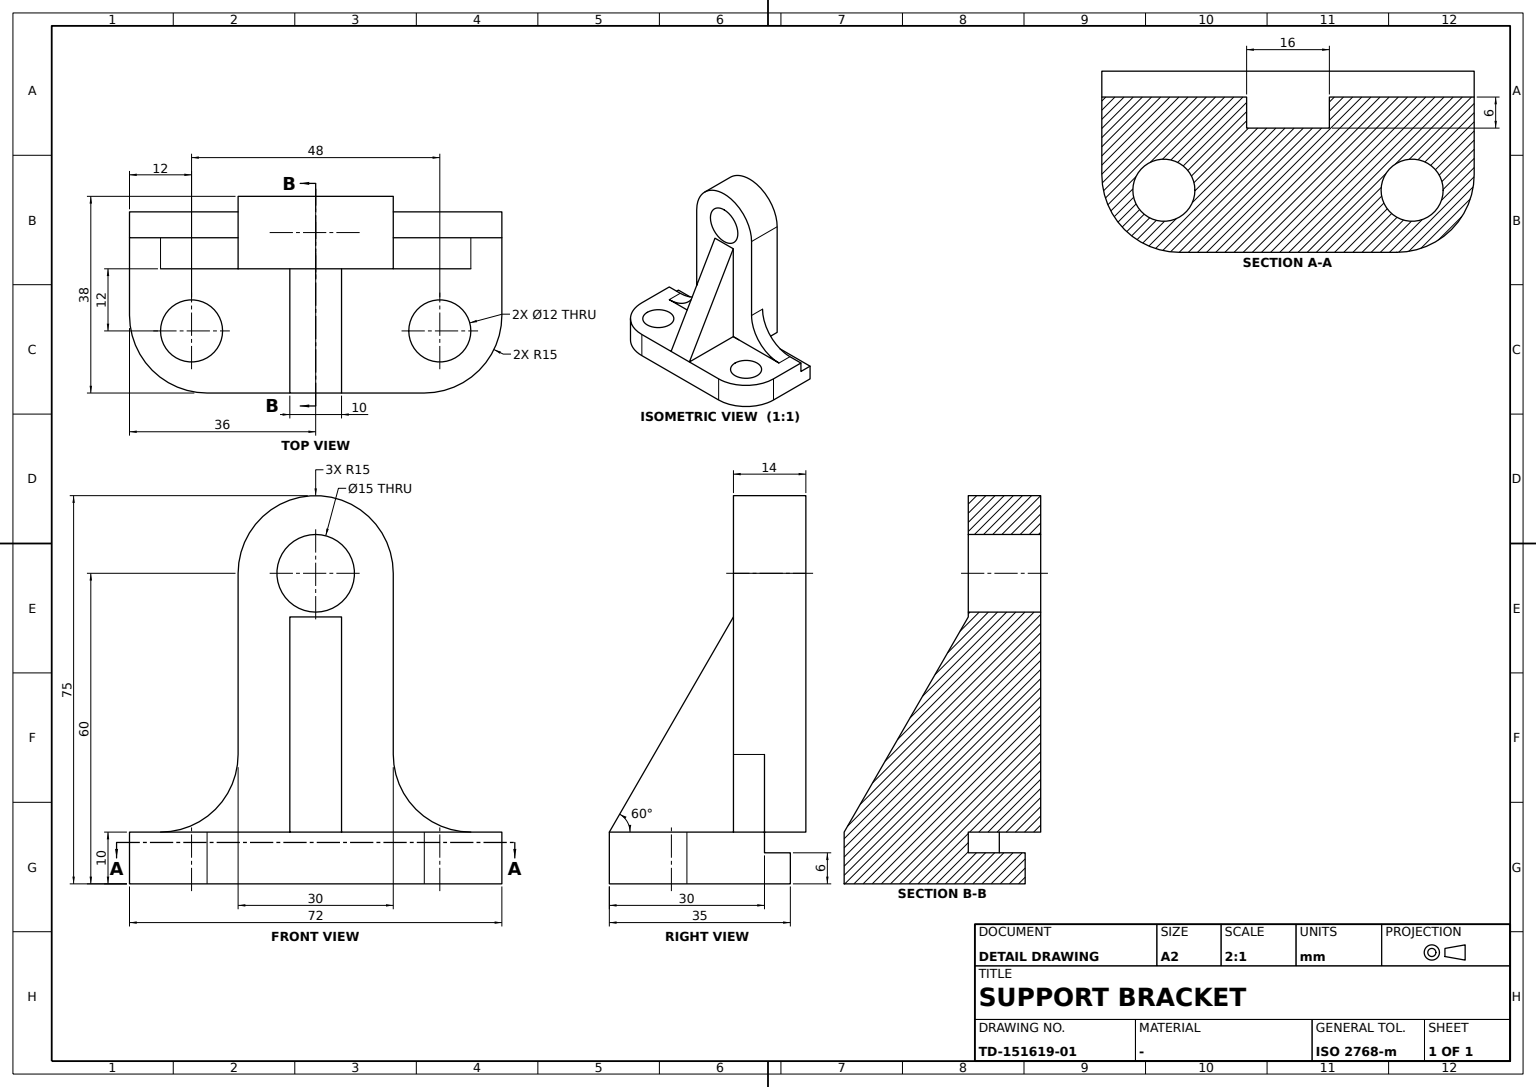
CATIA V5 part; units mm, degrees
sketch "Sketch1" plane through (0, 0, 0) normal (1, 0, 0) x (0, 1, 0)
  line L0 (-17.5, -5) -> (-17.5, 5)
  line L1 (-17.5, 5) -> (12.5, 5)
  line L2 (12.5, 5) -> (12.5, 1)
  line L3 (12.5, 1) -> (17.5, 1)
  line L4 (17.5, 1) -> (17.5, -5)
  line L5 (17.5, -5) -> (-17.5, -5)
  dimension "length L5" = 35
  dimension "length L4" = 6
  dimension "length L0" = 10
  dimension "length L3" = 5
  constraint vertical L0 y-axis
  constraint vertical L2 y-axis
  constraint vertical L4 y-axis
  constraint horizontal L1 x-axis
  constraint horizontal L3 x-axis
  constraint horizontal L5 x-axis
  constraint symmetry L1 L5 x-axis
  constraint symmetry L4 L0 y-axis
extrude "Pad1" add sketch "Sketch1" along normal mid plane 72
sketch "Sketch2" plane through (0, 12.5, 0) normal (0, 1, 0) x (-1, 0, 0)
  line L0 (-8, 5) -> (-8, 1)
  line L1 (-8, 1) -> (8, 1)
  line L2 (8, 1) -> (8, 5)
  line L3 (8, 5) -> (-8, 5)
  line L4 (36, 1) -> (-36, 1) construction
  line L5 (36, 5) -> (-36, 5) construction
  dimension "length L3" = 16
  constraint vertical L0 y-axis
  constraint vertical L2 y-axis
  constraint horizontal L1 x-axis
  constraint horizontal L3 x-axis
  constraint symmetry L2 L0 y-axis
  constraint coincidence L1 L4
  constraint coincidence L3 L5
extrude "Pocket1" cut sketch "Sketch2" against normal blind 6
sketch "Sketch3" plane through (0, 6.5, 0) normal (0, 1, 0) x (-1, 0, 0)
  arc A0 (15, 55) -> (-15, 55) centre (0, 55) ccw
  point P0 (0, 55)
  circle A1 centre (0, 55) radius 7.5
  line L0 (36, -5) -> (-36, -5) construction
  line L1 (-15, 55) -> (-15, 5)
  line L2 (-15, 5) -> (15, 5)
  line L3 (15, 5) -> (15, 55)
  line L4 (8, 5) -> (-8, 5) construction
  dimension "radius A0" = 15
  dimension "radius A1" = 7.5
  dimension "distance P0 L0" = 60
  constraint coincidence P0 y-axis
  constraint coincidence L2 L4
  constraint vertical L1 y-axis
  constraint vertical L3 y-axis
  constraint horizontal L2 x-axis
  constraint symmetry L1 L3 y-axis
  constraint tangency A0 L3
extrude "Pad2" add sketch "Sketch3" along normal blind 14
fillet "Fillet1" radius 15 2 edges at (15, 9.5, 5) (-15, 9.5, 5)
sketch "Sketch4" plane through (0, 0, 0) normal (1, 0, 0) x (0, 1, 0)
  line L0 (-17.5, 5) -> (6.5, 46.5692)
  point P0 (-17.5, 5)
  point P1 (6.5, 46.5692)
  point P2 (-17.5, 5)
  line L1 (-17.5, 5) -> (6.5, 5)
  point P3 (-17.5, 5)
  point P4 (6.5, 5)
  line L2 (6.5, 46.5692) -> (6.5, 5)
  point P5 (6.5, 5)
  point P6 (6.5, 46.5692)
  dimension "angle L0 L1" = 60
  constraint coincidence P0 P2
  constraint coincidence P5 L1
  constraint coincidence P5 P4
  constraint coincidence P3 P0
  constraint coincidence P1 P6
  constraint horizontal L1 x-axis
  constraint vertical L2 y-axis
extrude "Pad3" add sketch "Sketch4" along normal mid plane 10
fillet "Fillet2" radius 15 2 edges at (-36, -17.5, 0) (36, -17.5, 0)
sketch "Sketch5" plane through (0, 0, 5) normal (0, 0, 1) x (0, -1, 0)
  circle A0 centre (5.5, 24) radius 6
  point P0 (5.5, 24)
  line L0 (-17.5, -36) -> (-17.5, 36) construction
  circle A1 centre (5.5, -24) radius 6
  point P1 (5.5, -24)
  dimension "radius A0" = 6
  dimension "distance L0 P0" = 23
  dimension "radius A1" = 6
  dimension "distance P1 P0" = 48
  constraint symmetry P1 P0 x-axis
extrude "Pocket2" cut sketch "Sketch5" against normal through all
properties part number "v24"
